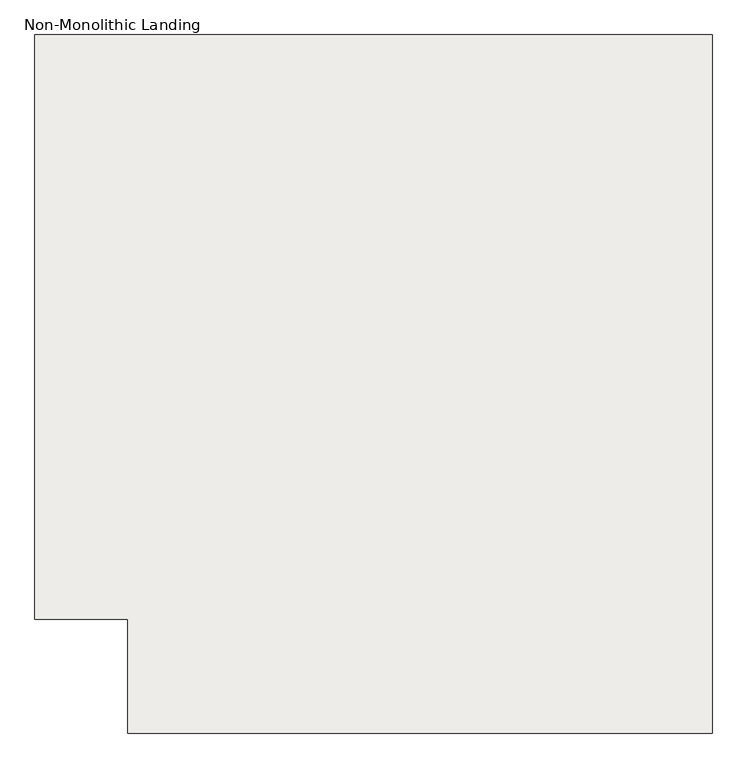
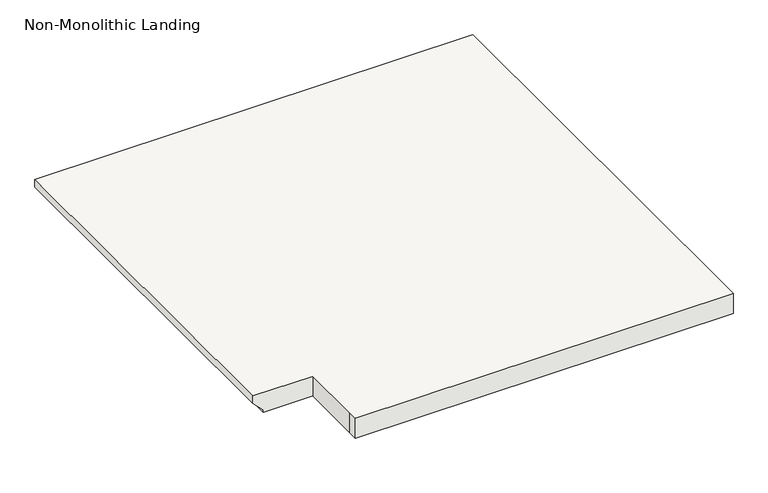
"""IFC4 building model written with IfcOpenShell, lengths in millimetres: slab geometry, Non-Monolithic Landing."""

from ifc_helpers import new_model, si_unit, origin, place, context, project, spatial, faceted_brep, source, transform, mapped, element, save


def non_monolithic_landing_bb3beaf2(model_context):
    return source(origin(), model_context, "Body", "Brep", [
        faceted_brep([(-11793.4585027, 10889.0453953, 2226.8447368), (-11793.4585027, 10889.0453953, 2245.8947368), (-11793.4585027, 11803.4453953, 2245.8947368), (-11793.4585027, 11803.4453953, 2226.8447368), (-11768.0585027, 10889.0453953, 2201.4447368), (-11768.0585027, 11803.4453953, 2201.4447368), (-11648.3149392, 10889.0453953, 2245.8947368), (-11648.3149392, 10736.3412275, 2245.8947368), (-11648.3149392, 10710.9412275, 2245.8947368), (-10733.9149392, 10710.9412275, 2245.8947368), (-10733.9149392, 10736.3412275, 2245.8947368), (-10733.9149392, 11803.4453953, 2245.8947368), (-11768.0585027, 10889.0453953, 2195.0947368), (-11768.0585027, 11803.4453953, 2195.0947368), (-10733.9149392, 11803.4453953, 2195.0947368), (-10733.9149392, 10736.3412275, 2195.0947368), (-10733.9149392, 10710.9412275, 2195.0947368), (-11648.3149392, 10710.9412275, 2195.0947368), (-11648.3149392, 10736.3412275, 2195.0947368), (-11648.3149392, 10889.0453953, 2195.0947368)], [[[0, 1, 2, 3]], [[4, 0, 3, 5]], [[6, 7, 8, 9, 10, 11, 2, 1]], [[12, 13, 14, 15, 16, 17, 18, 19]], [[13, 12, 4, 5]], [[6, 1, 0, 4, 12, 19]], [[7, 6, 19, 18]], [[8, 7, 18, 17]], [[9, 8, 17, 16]], [[10, 9, 16, 15]], [[11, 10, 15, 14]], [[2, 11, 14, 13, 5, 3]]]),
    ])


if __name__ == "__main__":
    model = new_model("IFC4")
    model_context = context("Model", 3, world=origin())
    ifc_project = project(units=[si_unit("LENGTHUNIT", "METRE", prefix="MILLI")], contexts=[model_context])
    site = spatial("IfcSite", under=ifc_project)
    building = spatial("IfcBuilding", under=site)
    placement = place(None, origin())
    non_monolithic_landing_shape = non_monolithic_landing_bb3beaf2(model_context)
    element("IfcSlab", 1, ObjectType="Non-Monolithic Landing", at=placement, inside=building, context=model_context, shape_type="MappedRepresentation", body=[
        mapped(non_monolithic_landing_shape, transform((0.0, 0.0, 0.0), x_axis=(1.0, 0.0, 0.0), y_axis=(0.0, 1.0, 0.0), z_axis=(0.0, 0.0, 1.0))),
    ])
    save(model, "model.ifc")
